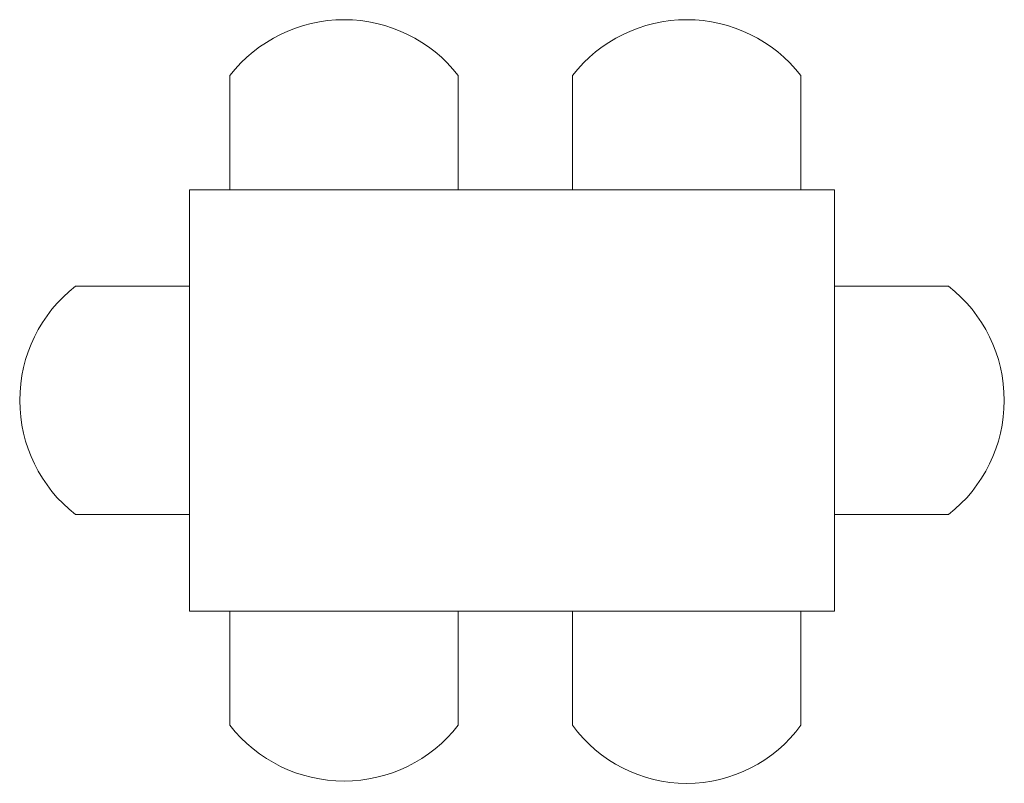
# Model space of a CAD drawing. Units: inches. Extents: x 2364 to 7426, y 1289 to 11972.
# Tile 6 of 6: x 6185 to 7426, y 11009 to 11972. Entities that reach past the tile are written whole.
import ezdxf

# ---------------------------------------------------------------- set-up
doc = ezdxf.new("R2010")
doc.units = ezdxf.units.IN
doc.layers.add('A-FURN', color=8, linetype='Continuous', lineweight=15)

# ---------------------------------------------------------------- blocks, each defined once
blk = doc.blocks.new('DINING TABLE')
for p, q in [((2443.51, 1632.65), (2443.51, 1644.65)), ((2467.51, 1632.65), (2467.51, 1644.65)), ((2479.51, 1632.65), (2479.51, 1644.65)), ((2503.51, 1632.65), (2503.51, 1644.65)), ((2427.28, 1622.52), (2439.28, 1622.52)), ((2507.03, 1622.52), (2519.03, 1622.52)), ((2427.28, 1598.52), (2439.28, 1598.52)), ((2507.03, 1598.52), (2519.03, 1598.52)), ((2443.51, 1576.39), (2443.51, 1588.39)), ((2467.51, 1576.39), (2467.51, 1588.39)), ((2479.51, 1576.39), (2479.51, 1588.39)), ((2503.51, 1576.39), (2503.51, 1588.39))]:
    blk.add_line(p, q)
blk.add_lwpolyline([(2439.28, 1632.65), (2507.03, 1632.65), (2507.03, 1588.39), (2439.28, 1588.39)], close=True)
for centre, radius, start, end in [((2455.51, 1635.3), 15.21, 37.9308, 142.0692), ((2491.51, 1635.3), 15.21, 37.9308, 142.0692), ((2436.64, 1610.52), 15.21, 127.9308, 232.0692), ((2509.67, 1610.52), 15.21, 307.9308, 52.0692), ((2455.51, 1585.74), 15.21, 217.9308, 322.0692), ((2491.51, 1585.15), 14.86, 216.1262, 323.8738)]:
    blk.add_arc(centre, radius, start, end)

msp = doc.modelspace()

# ---------------------------------------------------------------- block references
at = {"layer": 'A-FURN', "xscale": 12, "yscale": 12, "zscale": 12}
msp.add_blockref('DINING TABLE', (-22872.41, -7834.237), dxfattribs=at)

doc.saveas('drawing.dxf')
